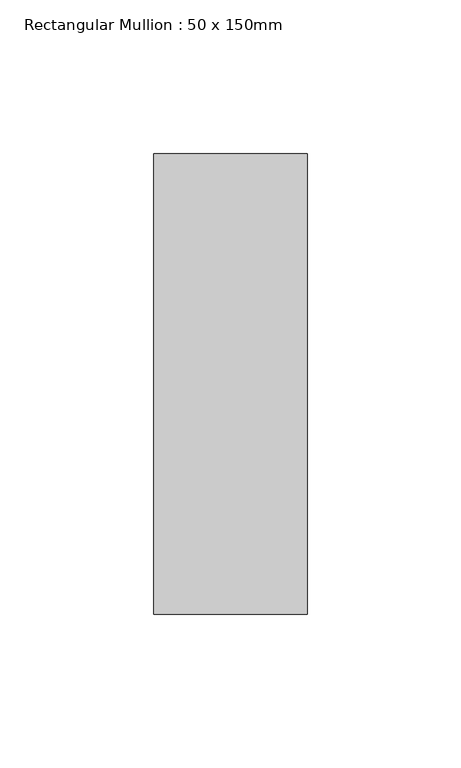
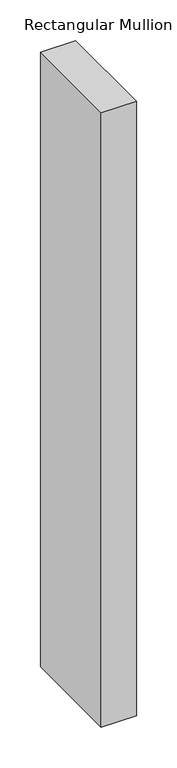
"""IFC4 building model written with IfcOpenShell, lengths in millimetres: member geometry, Rectangular Mullion : 50 x 150mm."""

from ifc_helpers import new_model, si_unit, frame, origin, place, context, project, spatial, polyline, outline, extrude, source, transform, mapped, element, save


def rectangular_mullion_50_x_150mm_116cff39(model_context):
    return source(origin(), model_context, "Body", "SweptSolid", [
        extrude(outline(polyline([(25.0, 75.0), (25.0, -75.0), (-25.0, -75.0), (-25.0, 75.0), (25.0, 75.0)])), frame((0.0, 0.0, -925.0), z_axis=(0.0, 0.0, 1.0), x_axis=(1.0, 0.0, 0.0)), (0.0, 0.0, 1.0), 925.0),
    ])


if __name__ == "__main__":
    model = new_model("IFC4")
    model_context = context("Model", 3, world=origin())
    ifc_project = project(units=[si_unit("LENGTHUNIT", "METRE", prefix="MILLI")], contexts=[model_context])
    site = spatial("IfcSite", under=ifc_project)
    building = spatial("IfcBuilding", under=site)
    placement = place(None, origin())
    rectangular_mullion_50_x_150mm_shape = rectangular_mullion_50_x_150mm_116cff39(model_context)
    element("IfcMember", 1, ObjectType="Rectangular Mullion : 50 x 150mm", at=placement, inside=building, context=model_context, shape_type="MappedRepresentation", body=[
        mapped(rectangular_mullion_50_x_150mm_shape, transform((0.0, 0.0, 0.0), x_axis=(1.0, 0.0, 0.0), y_axis=(0.0, 1.0, 0.0), z_axis=(0.0, 0.0, 1.0))),
    ])
    save(model, "model.ifc")

# Revit data of these elements
# Type "Rectangular Mullion : 50 x 150mm"
#   built-in parameter 1007304 = 0.492126 (stored number, unit not read)
#   built-in parameter 1007301 = 0.082021 (stored number, unit not read)
#   built-in parameter 1007300 = 0.082021 (stored number, unit not read)
# Element 1 (IfcMember, "Rectangular Mullion : 50 x 150mm")
#   Materials on its faces: "Aluminium"
# Materials
#   "Aluminium": class "Metal", colour RGB 247 247 247, transparency 0, Description = "Aluminium 6061", Cost = 0
